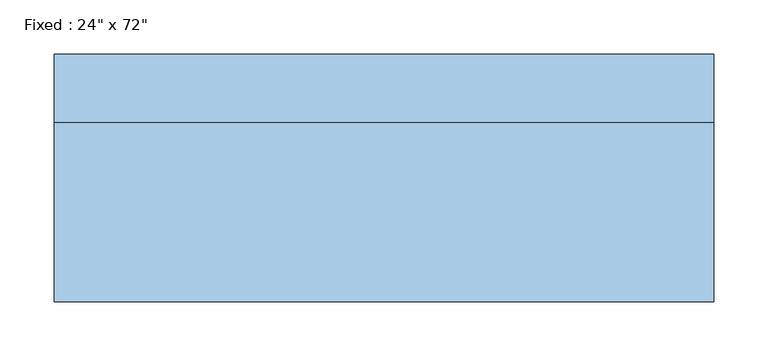
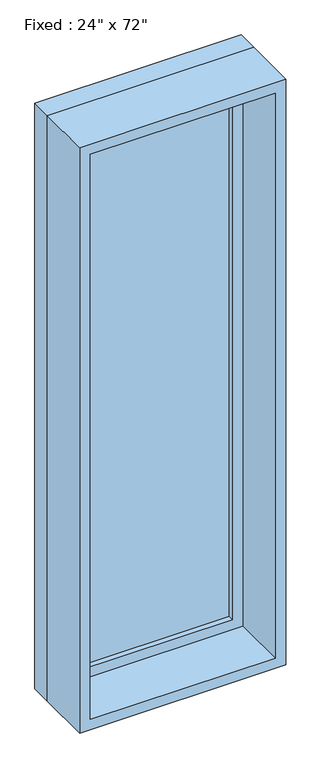
"""IFC4 building model written with IfcOpenShell, lengths in millimetres: window geometry."""

from ifc_helpers import new_model, si_unit, frame, origin, place, context, project, spatial, polyline, outline, extrude, source, transform, mapped, element, save


def window_fc882ab3(model_context):
    return source(origin(), model_context, "Body", "SweptSolid", [
        extrude(outline(polyline([(203.2, 66.675), (-279.4, 66.675), (-279.4, 79.375), (203.2, 79.375), (203.2, 66.675)])), frame((0.0, 0.0, 368.3), z_axis=(0.0, 0.0, 1.0), x_axis=(1.0, 0.0, 0.0)), (0.0, 0.0, 1.0), 1701.8),
        extrude(outline(polyline([(2114.55, -323.85), (323.85, -323.85), (323.85, 247.65), (2114.55, 247.65), (2114.55, -323.85)]), holes=[polyline([(2070.1, -279.4), (2070.1, 203.2), (368.3, 203.2), (368.3, -279.4), (2070.1, -279.4)])]), frame((0.0, 50.8, 0.0), z_axis=(0.0, 1.0, 0.0), x_axis=(0.0, 0.0, 1.0)), (0.0, 0.0, 1.0), 44.45),
        extrude(outline(polyline([(2133.6, -342.9), (304.8, -342.9), (304.8, 266.7), (2133.6, 266.7), (2133.6, -342.9)]), holes=[polyline([(2101.85, -311.15), (2101.85, 234.95), (336.55, 234.95), (336.55, -311.15), (2101.85, -311.15)])]), frame((0.0, -114.3, 0.0), z_axis=(0.0, 1.0, 0.0), x_axis=(0.0, 0.0, 1.0)), (0.0, 0.0, 1.0), 165.1),
        extrude(outline(polyline([(2133.6, 266.7), (2133.6, -342.9), (304.8, -342.9), (304.8, 266.7), (2133.6, 266.7)]), holes=[polyline([(2114.55, 247.65), (323.85, 247.65), (323.85, -323.85), (2114.55, -323.85), (2114.55, 247.65)])]), frame((0.0, 50.8, 0.0), z_axis=(0.0, 1.0, 0.0), x_axis=(0.0, 0.0, 1.0)), (0.0, 0.0, 1.0), 63.5),
    ])


if __name__ == "__main__":
    model = new_model("IFC4")
    model_context = context("Model", 3, world=origin())
    ifc_project = project(units=[si_unit("LENGTHUNIT", "METRE", prefix="MILLI")], contexts=[model_context])
    site = spatial("IfcSite", under=ifc_project)
    building = spatial("IfcBuilding", under=site)
    placement = place(None, origin())
    window_shape = window_fc882ab3(model_context)
    element("IfcWindow", 1, ObjectType="Fixed : 24\" x 72\"", at=placement, inside=building, context=model_context, shape_type="MappedRepresentation", body=[
        mapped(window_shape, transform((0.0, 0.0, 0.0), x_axis=(1.0, 0.0, 0.0), y_axis=(0.0, 1.0, 0.0), z_axis=(0.0, 0.0, 1.0))),
    ])
    save(model, "model.ifc")

# Revit data of these elements
# Type "Fixed : 24\" x 72\""
#   Type Mark = "7"
#   Construction Type Id = "GSP4R"
#   Assembly Code = "B2020100"
#   Analytic Construction = "1/8 in Pilkington single glazing"
#   Visual Light Transmittance = 0.9
#   Solar Heat Gain Coefficient = 0.78
#   Heat Transfer Coefficient (U) = 0.6496 BTU/(h·ft²·°F)
#   Height = 6' - 0"
#   Default Sill Height = 1' - 0"
#   Width = 2' - 0"
#   Window Inset = 0' - 0 3/4"
#   Define Thermal Properties by = 1
#   Define Thermal Properties by = 1
#   Glass Pane Material = Glass
#   Sash Material = Sash
#   Wall Closure = (empty or 0)
# Element 1 (IfcWindow, "Fixed : 24\" x 72\"")
#   Materials on its faces: "Sash", "Glass"
# Materials
#   "Glass": class "Glass", colour RGB 0 128 192, transparency 0.75, Description = "Soda Lime Glass", Cost = 0
#   "Sash": class "Wood", colour RGB 224 178 126, transparency 0, Cost = 0
